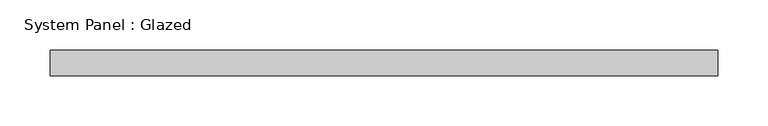
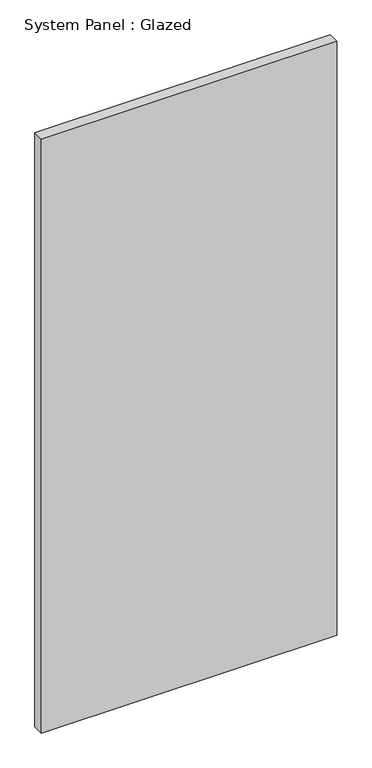
"""IFC4 building model written with IfcOpenShell, lengths in millimetres: plate geometry, System Panel : Glazed."""

from ifc_helpers import new_model, si_unit, origin, origin_with_axes, place, context, project, spatial, polyline, outline, extrude, source, transform, mapped, element, save


def system_panel_glazed_dae3c0ba(model_context):
    return source(origin(), model_context, "Body", "SweptSolid", [
        extrude(outline(polyline([(333.375, 19.05), (-333.375, 19.05), (-333.375, 44.45), (333.375, 44.45), (333.375, 19.05)])), origin_with_axes(), (0.0, 0.0, 1.0), 1417.4066766),
    ])


if __name__ == "__main__":
    model = new_model("IFC4")
    model_context = context("Model", 3, world=origin())
    ifc_project = project(units=[si_unit("LENGTHUNIT", "METRE", prefix="MILLI")], contexts=[model_context])
    site = spatial("IfcSite", under=ifc_project)
    building = spatial("IfcBuilding", under=site)
    placement = place(None, origin())
    system_panel_glazed_shape = system_panel_glazed_dae3c0ba(model_context)
    element("IfcPlate", 1, ObjectType="System Panel : Glazed", at=placement, inside=building, context=model_context, shape_type="MappedRepresentation", body=[
        mapped(system_panel_glazed_shape, transform((0.0, 0.0, 0.0), x_axis=(1.0, 0.0, 0.0), y_axis=(0.0, 1.0, 0.0), z_axis=(0.0, 0.0, 1.0))),
    ])
    save(model, "model.ifc")

# Revit data of these elements
# Type "System Panel : Glazed"
#   Construction Type Id = "GSP4R"
#   Analytic Construction = "1/8 in Pilkington single glazing"
#   Visual Light Transmittance = 0.9
#   Solar Heat Gain Coefficient = 0.86
#   Heat Transfer Coefficient (U) = 1.18115 BTU/(h·ft²·°F)
#   Define Thermal Properties by = 1
# Element 1 (IfcPlate, "System Panel : Glazed")
#   Materials on its faces: "Glass"
# Materials
#   "Glass": class "Glass", colour RGB 0 128 192, transparency 0.75, Description = "Soda Lime Glass", Cost = 0
